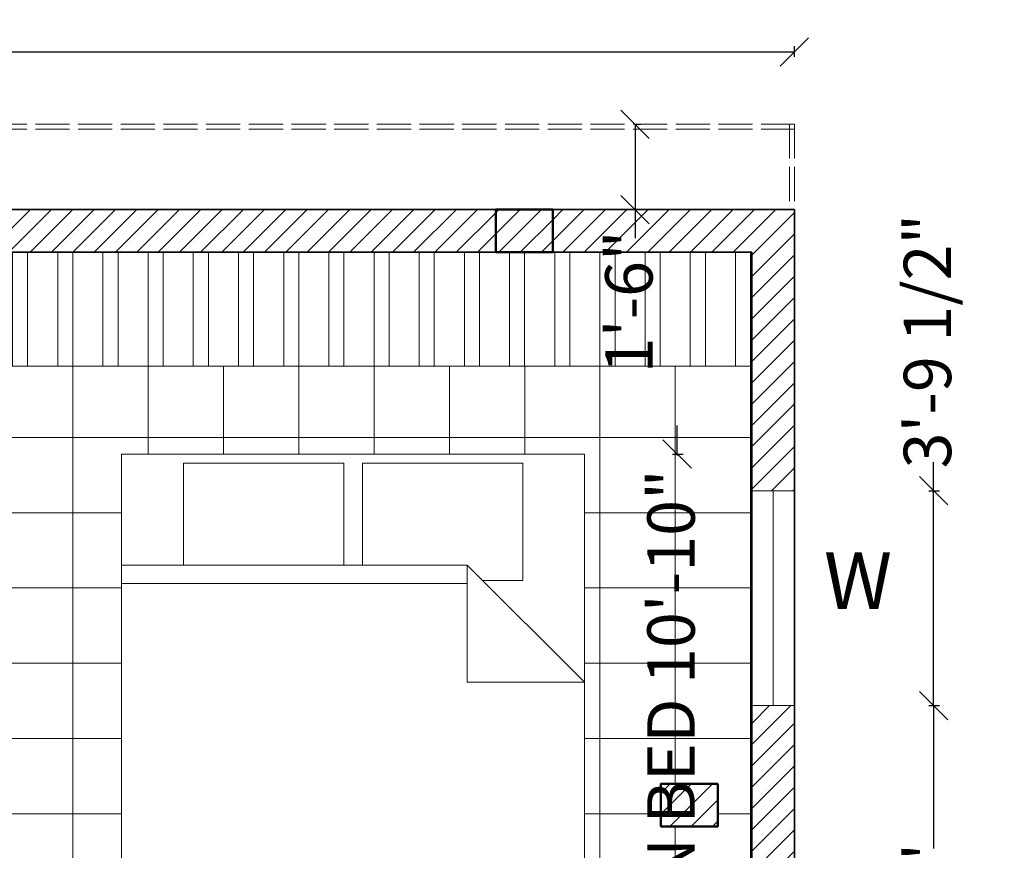
# Model space of a CAD drawing. Units: inches. Extents: x 2036 to 2670, y 319 to 920.
# Tile 15 of 15: x 2449 to 2657, y 723 to 898. Entities that reach past the tile are written whole.
import ezdxf

# ---------------------------------------------------------------- set-up
doc = ezdxf.new("R2010")
doc.units = ezdxf.units.IN
doc.linetypes.add('ACAD_ISO02W100', pattern=[15, 12, -3])
for name, color, linetype, lineweight in [('A-ANNO-DIMS', 2, 'Continuous', 18), ('A-ANNO-TEXT', 7, 'Continuous', 18), ('A-CASE', 7, 'Continuous', 18), ('A-CASE-PATT', 9, 'Continuous', 13), ('A-COLS', 7, 'Continuous', 50), ('A-FLOR-OVHD', 1, 'ACAD_ISO02W100', 13), ('A-FLOR-PATT', 8, 'Continuous', 9), ('A-FURN', 8, 'Continuous', 18), ('A-GLAZ', 4, 'Continuous', 18), ('A-WALL', 7, 'Continuous', 35)]:
    doc.layers.add(name, color=color, linetype=linetype, lineweight=lineweight)
doc.layers.add('A-COLS-PATT', color=240, linetype='Continuous', lineweight=13, true_color=0xed1f24)
doc.layers.add('A-WALL-PATT', color=52, linetype='Continuous', lineweight=13, true_color=0xc8c92d)
doc.styles.get("Standard").update_dxf_attribs({"font": 'arial.ttf'})
doc.dimstyles.new('ISO-25', dxfattribs={"dimtxt": 10, "dimasz": 6, "dimexe": 1.25, "dimexo": 0.625, "dimtad": 0, "dimdec": 1, "dimlunit": 3, "dimtxsty": 'Standard', "dimblk": 'OBLIQUE', "dimcen": 2.5, "dimclrd": 94, "dimclre": 94, "dimclrt": 1, "dimadec": 0, "dimazin": 0, "dimtfac": 1, "dimtdec": 1, "dimtmove": 0, "dimatfit": 3, "dimfxl": 1, "dimfxlon": 1, "dimarcsym": 0})

# ---------------------------------------------------------------- blocks, each defined once
blk = doc.blocks.new('Bed - Queen')
for p, q in [((0, -80.00003), (0, 0)), ((0, 0), (59.99999, 0)), ((59.99999, 0), (59.99999, -80.00003)), ((7.99999, -1.2), (28.79998, -1.2)), ((7.99999, -14.4), (7.99999, -1.2)), ((28.79998, -1.2), (28.79998, -14.4)), ((31.19999, -1.2), (51.99999, -1.2)), ((31.19999, -14.4), (31.19999, -1.2)), ((51.99999, -1.2), (51.99999, -16.4)), ((0, -14.4), (44.8, -14.4)), ((59.99999, -29.6), (44.8, -14.4)), ((44.8, -14.4), (44.8, -29.6)), ((51.99999, -16.4), (46.79936, -16.4)), ((44.8, -16.8), (0, -16.8)), ((44.8, -29.6), (59.99999, -29.6)), ((59.99999, -80.00003), (0, -80.00003))]:
    blk.add_line(p, q)
blk = doc.blocks.new('_Oblique')
at = {"color": 0, "linetype": 'ByBlock', "lineweight": -2}
blk.add_line((-0.5, -0.5), (0.5, 0.5), dxfattribs=at)
blk = doc.blocks.new('*D10')
at = {"layer": 'A-ANNO-DIMS', "color": 0, "lineweight": -2, "transparency": 16777216}
for p, q in [((2080.74, 889.93), (2080.74, 892.18)), ((2080.74, 890.93), (2328.73, 890.93)), ((2612.74, 890.93), (2364.74, 890.93)), ((2612.74, 889.93), (2612.74, 892.18))]:
    blk.add_line(p, q, dxfattribs=at)
at = {"layer": 'Defpoints', "color": 0, "transparency": 16777216}
for p in [(2612.74, 890.93), (2080.74, 875.68), (2612.74, 875.68)]:
    blk.add_point(p, dxfattribs=at)
at = {"layer": 'A-ANNO-DIMS', "color": 0, "lineweight": -2, "transparency": 16777216, "xscale": 6, "yscale": 6, "zscale": 6, "rotation": 180}
blk.add_blockref('_Oblique', (2080.74, 890.93), dxfattribs=at)
at = {"layer": 'A-ANNO-DIMS', "color": 0, "lineweight": -2, "transparency": 16777216, "xscale": 6, "yscale": 6, "zscale": 6}
blk.add_blockref('_Oblique', (2612.74, 890.93), dxfattribs=at)
at = {"layer": 'A-ANNO-DIMS', "color": 0, "transparency": 16777216, "insert": (2346.74, 890.93), "char_height": 10, "attachment_point": 5}
blk.add_mtext('44\'-4"', dxfattribs=at)
blk = doc.blocks.new('*D11')
at = {"layer": 'A-ANNO-DIMS', "color": 0, "lineweight": -2, "transparency": 16777216}
for p, q in [((2579.15, 875.68), (2580.4, 875.68)), ((2579.15, 875.68), (2579.15, 857.68)), ((2579.15, 857.68), (2580.4, 857.68)), ((2579.15, 857.68), (2579.15, 851.68))]:
    blk.add_line(p, q, dxfattribs=at)
at = {"layer": 'Defpoints', "color": 0, "transparency": 16777216}
for p in [(2578.53, 875.68), (2578.53, 857.68), (2579.15, 857.68)]:
    blk.add_point(p, dxfattribs=at)
at = {"layer": 'A-ANNO-DIMS', "color": 0, "lineweight": -2, "transparency": 16777216, "xscale": 6, "yscale": 6, "zscale": 6}
for p, rotation in [((2579.15, 875.68), 90), ((2579.15, 857.68), 270)]:
    blk.add_blockref('_Oblique', p, dxfattribs=dict(at, rotation=rotation))
at = {"layer": 'A-ANNO-DIMS', "color": 0, "transparency": 16777216, "insert": (2579.15, 838.24), "char_height": 10, "attachment_point": 5, "rotation": 90}
blk.add_mtext('1\'-6"', dxfattribs=at)
blk = doc.blocks.new('COL-9x12')
blk.add_lwpolyline([(9, 0), (0, 0), (0, 12), (9, 12)], close=True)
blk = doc.blocks.new('*D31')
at = {"layer": 'A-ANNO-DIMS', "color": 94, "lineweight": -2, "transparency": 16777216}
for p, q in [((2588.03, 806.13), (2588.03, 812.13)), ((2587.03, 806.13), (2589.28, 806.13)), ((2588.03, 806.13), (2588.03, 805.83)), ((2587.03, 676.01), (2589.28, 676.01)), ((2588.03, 676.01), (2588.03, 676.31)), ((2588.03, 676.01), (2588.03, 670.01))]:
    blk.add_line(p, q, dxfattribs=at)
at = {"layer": 'Defpoints', "color": 0, "transparency": 16777216}
for p in [(2568.52, 806.13), (2588.03, 806.13), (2568.52, 676.01)]:
    blk.add_point(p, dxfattribs=at)
at = {"layer": 'A-ANNO-DIMS', "color": 94, "lineweight": -2, "transparency": 16777216, "xscale": 6, "yscale": 6, "zscale": 6}
for p, rotation in [((2588.03, 806.13), 270), ((2588.03, 676.01), 90)]:
    blk.add_blockref('_Oblique', p, dxfattribs=dict(at, rotation=rotation))
at = {"layer": 'A-ANNO-DIMS', "color": 1, "transparency": 16777216, "insert": (2588.03, 741.07), "char_height": 10, "attachment_point": 5, "rotation": 90}
blk.add_mtext('QUEEN BED 10\'-10"', dxfattribs=at)
blk = doc.blocks.new('*D48')
at = {"layer": 'A-ANNO-DIMS', "color": 94, "lineweight": -2, "transparency": 16777216}
for p, q in [((2641.09, 753.07), (2643.34, 753.07)), ((2642.09, 753.07), (2642.09, 722.91)), ((2642.09, 665), (2642.09, 695.16)), ((2641.09, 665), (2643.34, 665))]:
    blk.add_line(p, q, dxfattribs=at)
at = {"layer": 'Defpoints', "color": 0, "transparency": 16777216}
for p in [(2612.74, 753.07), (2642.09, 753.07), (2612.74, 665)]:
    blk.add_point(p, dxfattribs=at)
at = {"layer": 'A-ANNO-DIMS', "color": 94, "lineweight": -2, "transparency": 16777216, "xscale": 6, "yscale": 6, "zscale": 6}
for p, rotation in [((2642.09, 753.07), 90), ((2642.09, 665), 270)]:
    blk.add_blockref('_Oblique', p, dxfattribs=dict(at, rotation=rotation))
at = {"layer": 'A-ANNO-DIMS', "color": 1, "transparency": 16777216, "insert": (2642.09, 709.03), "char_height": 10, "attachment_point": 5, "rotation": 90}
blk.add_mtext('7\'-4"', dxfattribs=at)
blk = doc.blocks.new('*D49')
at = {"layer": 'A-ANNO-DIMS', "color": 94, "lineweight": -2, "transparency": 16777216}
for p, q in [((2642.09, 798.38), (2642.09, 804.38)), ((2641.09, 798.38), (2643.34, 798.38)), ((2642.09, 753.07), (2642.09, 798.38)), ((2641.09, 753.07), (2643.34, 753.07))]:
    blk.add_line(p, q, dxfattribs=at)
at = {"layer": 'Defpoints', "color": 0, "transparency": 16777216}
for p in [(2612.74, 798.38), (2642.09, 798.38), (2612.74, 753.07)]:
    blk.add_point(p, dxfattribs=at)
at = {"layer": 'A-ANNO-DIMS', "color": 94, "lineweight": -2, "transparency": 16777216, "xscale": 6, "yscale": 6, "zscale": 6}
for p, rotation in [((2642.09, 798.38), 90), ((2642.09, 753.07), 270)]:
    blk.add_blockref('_Oblique', p, dxfattribs=dict(at, rotation=rotation))
at = {"layer": 'A-ANNO-DIMS', "color": 1, "transparency": 16777216, "insert": (2642.09, 829.94), "char_height": 10, "attachment_point": 5, "rotation": 90}
blk.add_mtext('3\'-9 1/2"', dxfattribs=at)

msp = doc.modelspace()

# ---------------------------------------------------------------- hatches: boundary and pattern name
at = {"layer": 'A-CASE-PATT'}
h = msp.add_hatch(dxfattribs=at)
h.set_pattern_fill('ANSI32', color=256, angle=45)
h.paths.add_polyline_path([(2603.74, 848.68), (2431.74, 848.68), (2431.74, 824.68), (2603.74, 824.68)])
at = {"layer": 'A-COLS-PATT'}
h = msp.add_hatch(dxfattribs=at)
h.set_pattern_fill('ANSI31', color=256)
h.paths.add_polyline_path([(2089.74, 875.68), (2080.74, 875.68), (2080.74, 863.68), (2089.74, 863.68)])
h.paths.add_polyline_path([(2089.74, 821.68), (2080.74, 821.68), (2080.74, 809.68), (2089.74, 809.68)])
h.paths.add_polyline_path([(2089.74, 624.2), (2080.74, 624.2), (2080.74, 612.2), (2089.74, 612.2)])
h.paths.add_polyline_path([(2158.74, 506.68), (2149.74, 506.68), (2149.74, 494.68), (2158.74, 494.68)])
h.paths.add_polyline_path([(2158.74, 617.33), (2149.74, 617.33), (2149.74, 605.33), (2158.74, 605.33)])
h.paths.add_polyline_path([(2158.74, 736.18), (2149.74, 736.18), (2149.74, 724.18), (2158.74, 724.18)])
h.paths.add_polyline_path([(2158.74, 852.81), (2149.74, 852.81), (2149.74, 843.81), (2158.74, 843.81)])
h.paths.add_polyline_path([(2161.74, 852.81), (2158.74, 852.81), (2158.74, 843.81), (2161.74, 843.81)])
h.paths.add_polyline_path([(2295.21, 857.66), (2290.74, 857.66), (2290.74, 848.68), (2295.21, 848.68)])
h.paths.add_polyline_path([(2290.74, 857.66), (2283.21, 857.66), (2283.21, 848.66), (2290.74, 848.66)])
h.paths.add_polyline_path([(2443.62, 857.68), (2431.62, 857.68), (2431.62, 848.68), (2443.62, 848.68)])
h.paths.add_polyline_path([(2561.81, 857.68), (2549.81, 857.68), (2549.81, 848.68), (2561.81, 848.68)])
h.paths.add_polyline_path([(2295.24, 737.65), (2290.74, 737.65), (2290.74, 728.68), (2295.24, 728.68)])
h.paths.add_polyline_path([(2309.27, 612.12), (2297.27, 612.12), (2297.27, 603.12), (2309.27, 603.12)])
h.paths.add_polyline_path([(2282.24, 503.68), (2270.24, 503.68), (2270.24, 494.68), (2282.24, 494.68)])
h.paths.add_polyline_path([(2431.74, 746.09), (2427.24, 746.09), (2427.24, 737.09), (2431.74, 737.09)])
h.paths.add_polyline_path([(2439.24, 746.09), (2431.74, 746.09), (2431.74, 737.09), (2439.24, 737.09)])
h.paths.add_polyline_path([(2596.59, 736.59), (2584.59, 736.59), (2584.59, 727.59), (2596.59, 727.59)])
h.paths.add_polyline_path([(2586.39, 623.71), (2574.39, 623.71), (2574.39, 619.18), (2586.39, 619.18)])
h.paths.add_polyline_path([(2586.39, 619.18), (2574.39, 619.18), (2574.39, 614.71), (2586.39, 614.71)])
h.paths.add_polyline_path([(2438.74, 623.68), (2431.24, 623.68), (2431.24, 619.18), (2438.74, 619.18)])
h.paths.add_polyline_path([(2438.74, 619.18), (2431.24, 619.18), (2431.24, 614.68), (2438.74, 614.68)])
h.paths.add_polyline_path([(2431.24, 623.68), (2426.74, 623.68), (2426.74, 614.68), (2431.24, 614.68), (2431.24, 619.18)])
h.paths.add_polyline_path([(2527.24, 503.68), (2515.24, 503.68), (2515.24, 494.68), (2527.24, 494.68)])
h.paths.add_polyline_path([(2590.31, 503.68), (2578.31, 503.68), (2578.31, 494.68), (2590.31, 494.68)])
at = {"layer": 'A-FLOR-PATT'}
h = msp.add_hatch(dxfattribs=at)
h.set_pattern_fill('ANSI31', color=256, scale=5, angle=135)
h.paths.add_polyline_path([(2290.74, 659.68), (2158.74, 659.68), (2158.74, 582.53), (2158.74, 545.51), (2158.74, 503.68), (2426.74, 503.68), (2426.74, 614.68), (2426.74, 623.68), (2426.74, 628.18), (2431.24, 628.18), (2431.24, 623.68), (2438.74, 623.68), (2438.74, 619.18), (2574.39, 619.18), (2574.39, 623.71), (2586.39, 623.71), (2586.39, 619.18), (2603.74, 619.18), (2603.74, 824.68), (2431.74, 824.68), (2431.74, 746.09), (2439.24, 746.09), (2439.24, 737.09), (2431.74, 737.09), (2431.74, 659.68), (2427.24, 659.68), (2427.24, 739.48), (2383.24, 739.48), (2383.24, 804.68), (2339.24, 804.68), (2339.24, 749.08), (2295.24, 749.08), (2295.24, 737.65), (2295.27, 737.65), (2295.27, 728.65), (2295.21, 728.65, -0.586418), (2272.74, 728.68), (2272.74, 824.68), (2270.11, 824.68), (2270.11, 829.18), (2290.74, 829.18), (2290.74, 848.66), (2283.21, 848.66), (2283.21, 857.66), (2289.74, 857.66), (2289.74, 874.68), (2158.74, 874.68), (2158.74, 852.81), (2161.74, 852.81), (2161.74, 843.81), (2158.74, 843.81), (2158.74, 829.18), (2224.74, 829.18), (2224.74, 800.68), (2182.74, 800.68), (2182.74, 733.41), (2158.74, 733.41), (2158.74, 728.68), (2235.24, 728.68), (2235.24, 714.81), (2230.74, 714.81), (2230.74, 724.18), (2158.74, 724.18), (2158.74, 664.18), (2230.74, 664.18), (2230.74, 678.81), (2235.24, 678.81), (2235.24, 664.18), (2290.74, 664.18)])
h.paths.add_polyline_path([(2309.27, 612.12), (2309.27, 603.12), (2297.27, 603.12), (2297.27, 612.12)], flags=16)
h.paths.add_polyline_path([(2280.12, 639.11), (2280.26, 638.18, -0.414214), (2279.26, 637.18), (2278.76, 637.18), (2279.26, 633.18), (2277.76, 633.18), (2277.26, 637.18), (2269.76, 637.18), (2262.26, 637.18), (2261.76, 633.18), (2260.26, 633.18), (2260.76, 637.18), (2260.26, 637.18, -0.414214), (2259.26, 638.18), (2259.41, 639.11, -0.541164), (2257.76, 641.18), (2260.76, 652.18), (2261.45, 652.18), (2261.53, 652.68), (2262.76, 652.68), (2262.25, 655.24, 0.001913), (2261.76, 655.18), (2259.76, 658.18, -0.15), (2279.76, 658.18), (2277.76, 655.18, 0.001913), (2277.27, 655.24), (2276.76, 652.68), (2278, 652.68), (2278.07, 652.18), (2278.76, 652.18), (2281.76, 641.18, -0.541163)], flags=16)
h.paths.add_polyline_path([(2245.98, 639.11), (2246.13, 638.18, -0.414214), (2245.13, 637.18), (2244.63, 637.18), (2245.13, 633.18), (2243.63, 633.18), (2243.13, 637.18), (2235.63, 637.18), (2228.13, 637.18), (2227.63, 633.18), (2226.13, 633.18), (2226.63, 637.18), (2226.13, 637.18, -0.414214), (2225.13, 638.18), (2225.27, 639.11, -0.541164), (2223.63, 641.18), (2226.63, 652.18), (2227.32, 652.18), (2227.39, 652.68), (2228.63, 652.68), (2228.12, 655.24, 0.001913), (2227.63, 655.18), (2225.63, 658.18, -0.15), (2245.63, 658.18), (2243.63, 655.18, 0.001913), (2243.14, 655.24), (2242.63, 652.68), (2243.86, 652.68), (2243.94, 652.18), (2244.63, 652.18), (2247.63, 641.18, -0.541163)], flags=16)
h.paths.add_polyline_path([(2351.59, 515.15, -0.151948), (2279.59, 515.15), (2279.59, 537.68), (2273.59, 537.68), (2273.59, 511.68, 0.190476), (2357.59, 511.68), (2357.59, 537.68), (2351.59, 537.68)])
h.paths.add_polyline_path([(2327.59, 536.13), (2327.59, 517.07), (2303.59, 517.07), (2303.59, 536.13)], flags=16)
h.paths.add_polyline_path([(2213.4, 639.11), (2213.55, 638.18, -0.414214), (2212.55, 637.18), (2212.05, 637.18), (2212.55, 633.18), (2211.05, 633.18), (2210.55, 637.18), (2203.05, 637.18), (2195.55, 637.18), (2195.05, 633.18), (2193.55, 633.18), (2194.05, 637.18), (2193.55, 637.18, -0.414214), (2192.55, 638.18), (2192.69, 639.11, -0.541164), (2191.05, 641.18), (2194.05, 652.18), (2194.73, 652.18), (2194.81, 652.68), (2196.05, 652.68), (2195.53, 655.24, 0.001913), (2195.05, 655.18), (2193.05, 658.18, -0.15), (2213.05, 658.18), (2211.05, 655.18, 0.001913), (2210.56, 655.24), (2210.05, 652.68), (2211.28, 652.68), (2211.36, 652.18), (2212.05, 652.18), (2215.05, 641.18, -0.541163)], flags=16)
h.paths.add_polyline_path([(2368.58, 538.02), (2370.52, 538.02), (2371.17, 532.84), (2380.89, 532.84), (2390.6, 532.84), (2391.25, 538.02), (2393.2, 538.02), (2392.55, 532.84), (2380.89, 532.84), (2368.58, 532.84, 0.414214), (2367.28, 531.54), (2367.47, 530.34, -0.483352), (2369.23, 527.65), (2371.82, 513.4), (2370.12, 513.4), (2370.22, 512.75), (2391.56, 512.75), (2391.66, 513.4), (2389.96, 513.4), (2392.55, 527.65, -1.387427), (2396.43, 527.65), (2392.55, 513.4), (2391.66, 513.4), (2391.56, 512.75), (2389.31, 512.75), (2390, 509.37, 0.003796), (2391.25, 509.51), (2393.84, 505.63, -0.15), (2367.93, 505.63), (2370.52, 509.51, 0.003901), (2371.81, 509.36), (2372.47, 512.75), (2370.22, 512.75), (2370.12, 513.4), (2369.23, 513.4), (2365.34, 527.65, -0.541163), (2367.47, 530.34), (2367.28, 531.54, -0.414214), (2368.58, 532.84), (2369.23, 532.84)])
h.paths.add_polyline_path([(2266.74, 538.02), (2266.09, 532.84), (2254.43, 532.84), (2242.12, 532.84, 0.414214), (2240.83, 531.54), (2241.01, 530.34, -0.483352), (2242.77, 527.65), (2245.36, 513.4), (2243.66, 513.4), (2243.76, 512.75), (2265.1, 512.75), (2265.2, 513.4), (2263.5, 513.4), (2266.09, 527.65, -1.387427), (2269.98, 527.65), (2266.09, 513.4), (2265.2, 513.4), (2265.1, 512.75), (2262.85, 512.75), (2263.54, 509.37, 0.003796), (2264.79, 509.51), (2267.39, 505.63, -0.15), (2241.47, 505.63), (2244.07, 509.51, 0.003901), (2245.36, 509.36), (2246.01, 512.75), (2243.76, 512.75), (2243.66, 513.4), (2242.77, 513.4), (2238.88, 527.65, -0.541163), (2241.01, 530.34), (2240.83, 531.54, -0.414214), (2242.12, 532.84), (2242.77, 532.84), (2242.12, 538.02), (2244.07, 538.02), (2244.71, 532.84), (2254.43, 532.84), (2264.15, 532.84), (2264.79, 538.02)])
h.paths.add_polyline_path([(2185.24, 620.36), (2185.24, 618.86), (2181.24, 618.36), (2181.24, 610.86), (2181.24, 603.36), (2185.24, 602.86), (2185.24, 601.36), (2181.24, 601.86), (2181.24, 601.36, -0.414214), (2180.24, 600.36), (2179.31, 600.5, -0.541164), (2177.24, 598.86), (2166.24, 601.86), (2166.24, 602.54), (2165.74, 602.62), (2165.74, 603.86), (2163.18, 603.34, 0.001913), (2163.24, 602.86), (2160.24, 600.86, -0.15), (2160.24, 620.86), (2163.24, 618.86, 0.001913), (2163.18, 618.37), (2165.74, 617.86), (2165.74, 619.09), (2166.24, 619.17), (2166.24, 619.86), (2177.24, 622.86, -0.541163), (2179.31, 621.21), (2180.24, 621.36, -0.414214), (2181.24, 620.36), (2181.24, 619.86)])
h.paths.add_polyline_path([(2470.92, 676.01), (2470.92, 806.13), (2568.52, 806.13), (2568.52, 676.01)], flags=16)
h.paths.add_polyline_path([(2177.74, 677.49), (2161.9, 677.49), (2161.9, 705.85), (2177.74, 705.85)], flags=16)
h.paths.add_polyline_path([(2176.74, 678.49), (2162.9, 678.49), (2162.9, 704.85), (2176.74, 704.85)], flags=0)
h.paths.add_polyline_path([(2175.01, 686.48), (2172.93, 686.48), (2172.93, 690.63), (2170.86, 690.63), (2170.86, 686.48), (2164.63, 686.48), (2164.63, 688.56), (2166.71, 688.56), (2168.78, 688.56), (2168.78, 690.63), (2164.63, 690.63), (2164.63, 696.85), (2166.71, 696.85), (2166.71, 692.71), (2168.78, 692.71), (2168.78, 696.85), (2175.01, 696.85), (2175.01, 694.78), (2170.86, 694.78), (2170.86, 692.71), (2175.01, 692.71)], flags=0)
h.paths.add_polyline_path([(2543.79, 782.71), (2483.94, 782.71), (2483.94, 804.18), (2517.77, 804.18), (2517.77, 782.71), (2521.67, 782.71), (2521.67, 804.18), (2555.5, 804.18), (2555.5, 779.45), (2547.05, 779.45), (2568.52, 757.98), (2543.79, 757.98)], flags=0)
h.paths.add_polyline_path([(2584.59, 727.59), (2584.59, 736.59), (2596.59, 736.59), (2596.59, 727.59)], flags=16)
h.paths.add_polyline_path([(2520.45, 647.03), (2553.79, 647.03), (2553.79, 658.23), (2520.45, 658.23)], flags=24)
h.paths.add_polyline_path([(2299.53, 573.74), (2331.71, 573.74), (2331.71, 584.94), (2299.53, 584.94)], flags=24)
h.paths.add_polyline_path([(2191.59, 685.19), (2212.12, 685.19), (2212.12, 696.38), (2191.59, 696.38)], flags=24)
h.paths.add_polyline_path([(2353.9, 649.86), (2379.08, 649.86), (2379.08, 661.06), (2353.9, 661.06)], flags=24)
h.paths.add_polyline_path([(2214.61, 763.31), (2237.46, 763.31), (2237.46, 779.56), (2214.61, 779.56)], flags=24)
h.paths.add_polyline_path([(2225.09, 819.31), (2269.29, 819.31), (2269.29, 844.04), (2225.09, 844.04)], flags=24)
h.paths.add_polyline_path([(2204.06, 845.04), (2226.92, 845.04), (2226.92, 856.24), (2204.06, 856.24)], flags=24)
h = msp.add_hatch(dxfattribs=at)
h.set_pattern_fill('ANSI31', color=256, scale=5, angle=45)
h.paths.add_polyline_path([(2290.74, 659.68), (2158.74, 659.68), (2158.74, 582.53), (2158.74, 545.51), (2158.74, 503.68), (2426.74, 503.68), (2426.74, 614.68), (2426.74, 623.68), (2426.74, 628.18), (2431.24, 628.18), (2431.24, 623.68), (2438.74, 623.68), (2438.74, 619.18), (2574.39, 619.18), (2574.39, 623.71), (2586.39, 623.71), (2586.39, 619.18), (2603.74, 619.18), (2603.74, 824.68), (2431.74, 824.68), (2431.74, 746.09), (2439.24, 746.09), (2439.24, 737.09), (2431.74, 737.09), (2431.74, 659.68), (2427.24, 659.68), (2427.24, 739.48), (2383.24, 739.48), (2383.24, 804.68), (2339.24, 804.68), (2339.24, 749.08), (2295.24, 749.08), (2295.24, 737.65), (2295.27, 737.65), (2295.27, 728.65), (2295.21, 728.65, -0.586418), (2272.74, 728.68), (2272.74, 824.68), (2270.11, 824.68), (2270.11, 829.18), (2290.74, 829.18), (2290.74, 848.66), (2283.21, 848.66), (2283.21, 857.66), (2289.74, 857.66), (2289.74, 874.68), (2158.74, 874.68), (2158.74, 852.81), (2161.74, 852.81), (2161.74, 843.81), (2158.74, 843.81), (2158.74, 829.18), (2224.74, 829.18), (2224.74, 800.68), (2182.74, 800.68), (2182.74, 733.41), (2158.74, 733.41), (2158.74, 728.68), (2235.24, 728.68), (2235.24, 714.81), (2230.74, 714.81), (2230.74, 724.18), (2158.74, 724.18), (2158.74, 664.18), (2230.74, 664.18), (2230.74, 678.81), (2235.24, 678.81), (2235.24, 664.18), (2290.74, 664.18)])
h.paths.add_polyline_path([(2309.27, 612.12), (2309.27, 603.12), (2297.27, 603.12), (2297.27, 612.12)], flags=16)
h.paths.add_polyline_path([(2280.12, 639.11), (2280.26, 638.18, -0.414214), (2279.26, 637.18), (2278.76, 637.18), (2279.26, 633.18), (2277.76, 633.18), (2277.26, 637.18), (2269.76, 637.18), (2262.26, 637.18), (2261.76, 633.18), (2260.26, 633.18), (2260.76, 637.18), (2260.26, 637.18, -0.414214), (2259.26, 638.18), (2259.41, 639.11, -0.541164), (2257.76, 641.18), (2260.76, 652.18), (2261.45, 652.18), (2261.53, 652.68), (2262.76, 652.68), (2262.25, 655.24, 0.001913), (2261.76, 655.18), (2259.76, 658.18, -0.15), (2279.76, 658.18), (2277.76, 655.18, 0.001913), (2277.27, 655.24), (2276.76, 652.68), (2278, 652.68), (2278.07, 652.18), (2278.76, 652.18), (2281.76, 641.18, -0.541163)], flags=16)
h.paths.add_polyline_path([(2245.98, 639.11), (2246.13, 638.18, -0.414214), (2245.13, 637.18), (2244.63, 637.18), (2245.13, 633.18), (2243.63, 633.18), (2243.13, 637.18), (2235.63, 637.18), (2228.13, 637.18), (2227.63, 633.18), (2226.13, 633.18), (2226.63, 637.18), (2226.13, 637.18, -0.414214), (2225.13, 638.18), (2225.27, 639.11, -0.541164), (2223.63, 641.18), (2226.63, 652.18), (2227.32, 652.18), (2227.39, 652.68), (2228.63, 652.68), (2228.12, 655.24, 0.001913), (2227.63, 655.18), (2225.63, 658.18, -0.15), (2245.63, 658.18), (2243.63, 655.18, 0.001913), (2243.14, 655.24), (2242.63, 652.68), (2243.86, 652.68), (2243.94, 652.18), (2244.63, 652.18), (2247.63, 641.18, -0.541163)], flags=16)
h.paths.add_polyline_path([(2351.59, 537.68), (2351.59, 515.15, -0.151948), (2279.59, 515.15), (2279.59, 537.68), (2273.59, 537.68), (2273.59, 511.68, 0.190476), (2357.59, 511.68), (2357.59, 537.68)])
h.paths.add_polyline_path([(2368.58, 538.02), (2370.52, 538.02), (2371.17, 532.84), (2380.89, 532.84), (2390.6, 532.84), (2391.25, 538.02), (2393.2, 538.02), (2392.55, 532.84), (2380.89, 532.84), (2368.58, 532.84, 0.414214), (2367.28, 531.54), (2367.47, 530.34, -0.483352), (2369.23, 527.65), (2371.82, 513.4), (2370.12, 513.4), (2370.22, 512.75), (2391.56, 512.75), (2391.66, 513.4), (2389.96, 513.4), (2392.55, 527.65, -1.387427), (2396.43, 527.65), (2392.55, 513.4), (2391.66, 513.4), (2391.56, 512.75), (2389.31, 512.75), (2390, 509.37, 0.003796), (2391.25, 509.51), (2393.84, 505.63, -0.15), (2367.93, 505.63), (2370.52, 509.51, 0.003901), (2371.81, 509.36), (2372.47, 512.75), (2370.22, 512.75), (2370.12, 513.4), (2369.23, 513.4), (2365.34, 527.65, -0.541163), (2367.47, 530.34), (2367.28, 531.54, -0.414214), (2368.58, 532.84), (2369.23, 532.84)])
h.paths.add_polyline_path([(2327.59, 536.13), (2327.59, 517.07), (2303.59, 517.07), (2303.59, 536.13)], flags=16)
h.paths.add_polyline_path([(2470.92, 676.01), (2470.92, 806.13), (2568.52, 806.13), (2568.52, 676.01)], flags=16)
h.paths.add_polyline_path([(2266.74, 538.02), (2266.09, 532.84), (2254.43, 532.84), (2242.12, 532.84, 0.414214), (2240.83, 531.54), (2241.01, 530.34, -0.483352), (2242.77, 527.65), (2245.36, 513.4), (2243.66, 513.4), (2243.76, 512.75), (2265.1, 512.75), (2265.2, 513.4), (2263.5, 513.4), (2266.09, 527.65, -1.387427), (2269.98, 527.65), (2266.09, 513.4), (2265.2, 513.4), (2265.1, 512.75), (2262.85, 512.75), (2263.54, 509.37, 0.003796), (2264.79, 509.51), (2267.39, 505.63, -0.15), (2241.47, 505.63), (2244.07, 509.51, 0.003901), (2245.36, 509.36), (2246.01, 512.75), (2243.76, 512.75), (2243.66, 513.4), (2242.77, 513.4), (2238.88, 527.65, -0.541163), (2241.01, 530.34), (2240.83, 531.54, -0.414214), (2242.12, 532.84), (2242.77, 532.84), (2242.12, 538.02), (2244.07, 538.02), (2244.71, 532.84), (2254.43, 532.84), (2264.15, 532.84), (2264.79, 538.02)])
h.paths.add_polyline_path([(2213.4, 639.11), (2213.55, 638.18, -0.414214), (2212.55, 637.18), (2212.05, 637.18), (2212.55, 633.18), (2211.05, 633.18), (2210.55, 637.18), (2203.05, 637.18), (2195.55, 637.18), (2195.05, 633.18), (2193.55, 633.18), (2194.05, 637.18), (2193.55, 637.18, -0.414214), (2192.55, 638.18), (2192.69, 639.11, -0.541164), (2191.05, 641.18), (2194.05, 652.18), (2194.73, 652.18), (2194.81, 652.68), (2196.05, 652.68), (2195.53, 655.24, 0.001913), (2195.05, 655.18), (2193.05, 658.18, -0.15), (2213.05, 658.18), (2211.05, 655.18, 0.001913), (2210.56, 655.24), (2210.05, 652.68), (2211.28, 652.68), (2211.36, 652.18), (2212.05, 652.18), (2215.05, 641.18, -0.541163)], flags=16)
h.paths.add_polyline_path([(2185.24, 620.36), (2185.24, 618.86), (2181.24, 618.36), (2181.24, 610.86), (2181.24, 603.36), (2185.24, 602.86), (2185.24, 601.36), (2181.24, 601.86), (2181.24, 601.36, -0.414214), (2180.24, 600.36), (2179.31, 600.5, -0.541164), (2177.24, 598.86), (2166.24, 601.86), (2166.24, 602.54), (2165.74, 602.62), (2165.74, 603.86), (2163.18, 603.34, 0.001913), (2163.24, 602.86), (2160.24, 600.86, -0.15), (2160.24, 620.86), (2163.24, 618.86, 0.001913), (2163.18, 618.37), (2165.74, 617.86), (2165.74, 619.09), (2166.24, 619.17), (2166.24, 619.86), (2177.24, 622.86, -0.541163), (2179.31, 621.21), (2180.24, 621.36, -0.414214), (2181.24, 620.36), (2181.24, 619.86)])
h.paths.add_polyline_path([(2177.74, 677.49), (2161.9, 677.49), (2161.9, 705.85), (2177.74, 705.85)], flags=16)
h.paths.add_polyline_path([(2176.74, 678.49), (2162.9, 678.49), (2162.9, 704.85), (2176.74, 704.85)], flags=0)
h.paths.add_polyline_path([(2175.01, 686.48), (2172.93, 686.48), (2172.93, 690.63), (2170.86, 690.63), (2170.86, 686.48), (2164.63, 686.48), (2164.63, 688.56), (2166.71, 688.56), (2168.78, 688.56), (2168.78, 690.63), (2164.63, 690.63), (2164.63, 696.85), (2166.71, 696.85), (2166.71, 692.71), (2168.78, 692.71), (2168.78, 696.85), (2175.01, 696.85), (2175.01, 694.78), (2170.86, 694.78), (2170.86, 692.71), (2175.01, 692.71)], flags=0)
h.paths.add_polyline_path([(2543.79, 782.71), (2483.94, 782.71), (2483.94, 804.18), (2517.77, 804.18), (2517.77, 782.71), (2521.67, 782.71), (2521.67, 804.18), (2555.5, 804.18), (2555.5, 779.45), (2547.05, 779.45), (2568.52, 757.98), (2543.79, 757.98)], flags=0)
h.paths.add_polyline_path([(2584.59, 727.59), (2584.59, 736.59), (2596.59, 736.59), (2596.59, 727.59)], flags=16)
h.paths.add_polyline_path([(2520.45, 647.03), (2553.79, 647.03), (2553.79, 658.23), (2520.45, 658.23)], flags=24)
h.paths.add_polyline_path([(2299.53, 573.74), (2331.71, 573.74), (2331.71, 584.94), (2299.53, 584.94)], flags=24)
h.paths.add_polyline_path([(2191.59, 685.19), (2212.12, 685.19), (2212.12, 696.38), (2191.59, 696.38)], flags=24)
h.paths.add_polyline_path([(2353.9, 649.86), (2379.08, 649.86), (2379.08, 661.06), (2353.9, 661.06)], flags=24)
h.paths.add_polyline_path([(2214.61, 763.31), (2237.46, 763.31), (2237.46, 779.56), (2214.61, 779.56)], flags=24)
h.paths.add_polyline_path([(2225.09, 819.31), (2269.29, 819.31), (2269.29, 844.04), (2225.09, 844.04)], flags=24)
h.paths.add_polyline_path([(2204.06, 845.04), (2226.92, 845.04), (2226.92, 856.24), (2204.06, 856.24)], flags=24)
at = {"layer": 'A-WALL-PATT'}
h = msp.add_hatch(dxfattribs=at)
h.set_pattern_fill('ANSI31', color=256)
h.paths.add_polyline_path([(2089.74, 863.68), (2080.74, 863.68), (2080.74, 821.68), (2089.74, 821.68)])
h.paths.add_polyline_path([(2089.74, 809.68), (2080.74, 809.68), (2080.74, 624.2), (2089.74, 624.2), (2089.74, 707.68), (2089.74, 767.68)])
h.paths.add_polyline_path([(2149.74, 818.68), (2089.74, 818.68), (2089.74, 809.68), (2149.74, 809.68)])
h.paths.add_polyline_path([(2158.74, 875.68), (2089.74, 875.68), (2089.74, 866.68), (2149.74, 866.68), (2149.74, 852.81), (2158.74, 852.81)])
h.paths.add_polyline_path([(2158.74, 843.81), (2149.74, 843.81), (2149.74, 736.18), (2158.74, 736.18), (2158.74, 824.68)])
h.paths.add_polyline_path([(2181.31, 829.18), (2158.74, 829.18), (2158.74, 824.68), (2181.31, 824.68)])
h.paths.add_polyline_path([(2224.74, 829.18), (2212.72, 829.18), (2212.72, 824.68), (2224.74, 824.68)])
h.paths.add_polyline_path([(2177.02, 503.68), (2158.74, 503.68), (2158.74, 494.68), (2177.02, 494.68)])
h.paths.add_polyline_path([(2158.74, 664.18), (2158.74, 680.02), (2149.74, 680.02), (2149.74, 617.33), (2158.74, 617.33)])
h.paths.add_polyline_path([(2158.74, 724.18), (2149.74, 724.18), (2149.74, 704.02), (2158.74, 704.02)])
h.paths.add_polyline_path([(2235.24, 728.68), (2158.74, 728.68), (2158.74, 724.18), (2230.74, 724.18), (2230.74, 714.81), (2235.24, 714.81)])
h.paths.add_polyline_path([(2290.74, 664.18), (2235.24, 664.18), (2235.24, 678.81), (2230.74, 678.81), (2230.74, 664.18), (2158.74, 664.18), (2158.74, 659.68), (2290.74, 659.68)])
h.paths.add_polyline_path([(2270.24, 503.68), (2227.17, 503.68), (2227.17, 494.68), (2270.24, 494.68)])
h.paths.add_polyline_path([(2515.24, 503.68), (2380.89, 503.68), (2380.89, 494.68), (2515.24, 494.68)])
h.paths.add_polyline_path([(2292.21, 503.68), (2282.24, 503.68), (2282.24, 494.68), (2292.21, 494.68)])
h.paths.add_polyline_path([(2578.31, 503.68), (2527.24, 503.68), (2527.24, 494.68), (2578.31, 494.68)])
h.paths.add_polyline_path([(2603.74, 503.68), (2590.31, 503.68), (2590.31, 494.68), (2603.74, 494.68)])
h.paths.add_polyline_path([(2612.74, 503.68), (2603.74, 503.68), (2603.74, 494.68), (2612.74, 494.68)])
h.paths.add_polyline_path([(2549.81, 857.68), (2443.62, 857.68), (2443.62, 848.68), (2549.81, 848.68)])
h.paths.add_polyline_path([(2295.24, 848.66), (2290.74, 848.66), (2290.74, 829.18), (2270.11, 829.18), (2270.11, 824.68), (2290.74, 824.68), (2290.74, 737.65), (2295.24, 737.65)])
h.paths.add_polyline_path([(2431.74, 737.09), (2427.24, 737.09), (2427.24, 659.68), (2431.74, 659.68)])
h.paths.add_polyline_path([(2431.74, 848.68), (2427.24, 848.68), (2427.24, 746.09), (2431.74, 746.09)])
h.paths.add_polyline_path([(2574.39, 619.18), (2495.46, 619.18), (2495.46, 614.68), (2574.39, 614.68)])
h.paths.add_polyline_path([(2461.84, 619.18), (2438.74, 619.18), (2438.74, 614.68), (2461.84, 614.68)])
h.paths.add_polyline_path([(2603.74, 619.18), (2586.39, 619.18), (2586.39, 614.68), (2603.74, 614.68)], flags=17)
h = msp.add_hatch(dxfattribs=at)
h.set_pattern_fill('ANSI31', color=256)
h.paths.add_polyline_path([(2561.81, 857.68), (2561.81, 848.68), (2603.74, 848.68), (2603.74, 798.38), (2612.74, 798.38), (2612.74, 857.68)])
h.paths.add_polyline_path([(2603.74, 665), (2612.74, 665), (2612.74, 753.07), (2603.74, 753.07)])
h.paths.add_polyline_path([(2612.74, 623.23), (2603.74, 623.23), (2603.74, 614.68), (2603.74, 577.61), (2612.74, 577.61)])
h.paths.add_polyline_path([(2612.74, 553.61), (2603.74, 553.61), (2603.74, 503.68), (2612.74, 503.68)])

# ---------------------------------------------------------------- linework, layer by layer
at = {"layer": 'A-CASE'}
msp.add_line((2603.74, 824.68), (2431.74, 824.68), dxfattribs=at)
at = {"layer": 'A-FLOR-OVHD', "ltscale": 0.6}
for p, q in [((2290.74, 875.68), (2612.74, 875.68)), ((2290.74, 874.68), (2612.74, 874.68)), ((2611.74, 875.68), (2611.74, 857.68)), ((2612.74, 875.68), (2612.74, 857.68))]:
    msp.add_line(p, q, dxfattribs=at)
at = {"layer": 'A-GLAZ'}
for p, q in [((2603.74, 798.38), (2612.74, 798.38)), ((2608.24, 798.38), (2608.24, 753.07)), ((2603.74, 753.07), (2612.74, 753.07))]:
    msp.add_line(p, q, dxfattribs=at)
at = {"layer": 'A-WALL'}
for p, q in [((2612.74, 857.68), (2290.74, 857.68)), ((2612.74, 494.13), (2612.74, 857.68)), ((2603.74, 848.68), (2431.74, 848.68)), ((2603.74, 614.68), (2603.74, 848.68))]:
    msp.add_line(p, q, dxfattribs=at)

# ---------------------------------------------------------------- block references
at = {"layer": 'A-COLS'}
for p, rotation in [((2561.81, 848.68), 89.9999999999986), ((2596.59, 727.59), 89.9999999999968)]:
    msp.add_blockref('COL-9x12', p, dxfattribs=dict(at, rotation=rotation))
at = {"layer": 'A-FURN', "xscale": 1.626514147143349, "yscale": 1.626514147143349, "zscale": 1.626514147143349}
msp.add_blockref('Bed - Queen', (2470.92, 806.13), dxfattribs=at)

# ---------------------------------------------------------------- texts
at = {"layer": 'A-ANNO-TEXT', "insert": (2618.97, 785.42), "char_height": 12, "attachment_point": 1}
msp.add_mtext_dynamic_manual_height_columns('W', width=27.6972, gutter_width=12.5, heights=[0], dxfattribs=at)

# ---------------------------------------------------------------- dimensions: what is measured, and where the dimension line sits
at = {"layer": 'A-ANNO-DIMS'}
dim = msp.add_linear_dim(base=(2612.74, 890.93), p1=(2080.74, 875.68), p2=(2612.74, 875.68), dimstyle='ISO-25', override={"dimclrd": 0, "dimclre": 0, "dimclrt": 0}, dxfattribs=at)
dim.commit()
dim.dimension.update_dxf_attribs({"geometry": '*D10', "text_midpoint": (2346.74, 890.93)})
for base, p1, p2, override, picture, middle in [((2579.15, 857.68), (2578.53, 875.68), (2578.53, 857.68), {"dimclrd": 0, "dimclre": 0, "dimclrt": 0}, '*D11', (2579.15, 838.24)), ((2642.09, 798.38), (2612.74, 753.07), (2612.74, 798.38), {"dimdec": 1, "dimlfac": 1, "dimrnd": 0, "dimzin": 1, "dimdsep": 46, "dimlunit": 4, "dimfrac": 2}, '*D49', (2642.09, 829.94)), ((2642.09, 753.07), (2612.74, 665), (2612.74, 753.07), {"dimdec": 1, "dimlfac": 1, "dimrnd": 0, "dimzin": 1, "dimdsep": 46, "dimlunit": 4, "dimfrac": 2}, '*D48', (2642.09, 709.03))]:
    dim = msp.add_linear_dim(base=base, p1=p1, p2=p2, angle=90, dimstyle='ISO-25', override=override, dxfattribs=at)
    dim.commit()
    dim.dimension.update_dxf_attribs({"geometry": picture, "text_midpoint": middle})
dim = msp.add_linear_dim(base=(2588.03, 806.13), p1=(2568.52, 676.01), p2=(2568.52, 806.13), angle=90, text='QUEEN BED <>', dimstyle='ISO-25', override={"dimdec": 1, "dimlfac": 1, "dimrnd": 0, "dimzin": 1, "dimdsep": 46, "dimlunit": 4, "dimfrac": 2}, dxfattribs=at)
dim.commit()
dim.dimension.update_dxf_attribs({"geometry": '*D31', "text_midpoint": (2588.03, 741.07)})

doc.saveas('drawing.dxf')
